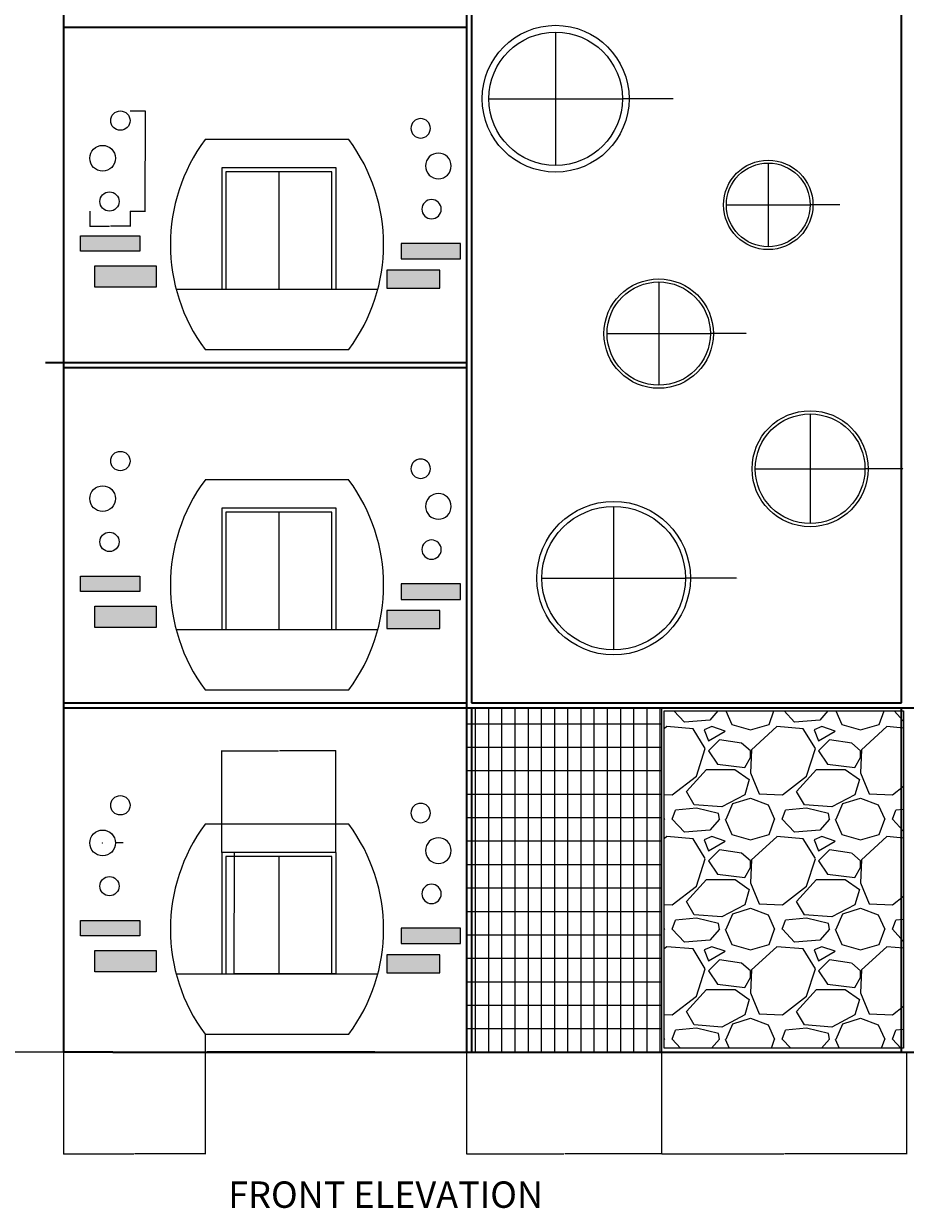
# Model space of a CAD drawing. Units: inches. Extents: x 328 to 2318, y 647 to 2548.
# Tile 2 of 5: x 1040 to 1841, y 647 to 1724. Entities that reach past the tile are written whole.
import ezdxf

# ---------------------------------------------------------------- set-up
doc = ezdxf.new("R2010")
doc.units = ezdxf.units.IN
doc.header["$MEASUREMENT"] = 0
for name, color, linetype, lineweight in [('A-ANNO-DIMS', 2, 'Continuous', 18), ('A-ANNO-TEXT', 7, 'Continuous', 25), ('A-ELEV', 7, 'Continuous', 35), ('A-ELEV-CLAD', 7, 'Continuous', 25), ('A-ELEV-ORNM', 7, 'Continuous', 18), ('A-ELEV-PATT', 8, 'Continuous', 13), ('A-GLAZ', 4, 'Continuous', 25)]:
    doc.layers.add(name, color=color, linetype=linetype, lineweight=lineweight)
doc.layers.add('A-ELEV-ORNM-PATT', color=18, linetype='Continuous', lineweight=13, true_color=0x000000)
doc.styles.get("Standard").update_dxf_attribs({"font": 'arial.ttf'})
doc.dimstyles.get("Standard").update_dxf_attribs({"dimtxt": 0.18, "dimasz": 0.18, "dimexe": 0.18, "dimexo": 0.0625, "dimgap": 0.09, "dimtad": 0, "dimtih": 1, "dimtoh": 1, "dimdec": 4, "dimzin": 0, "dimdsep": 46, "dimtxsty": 'Standard', "dimcen": 0.09, "dimadec": 0, "dimazin": 0, "dimtfac": 1, "dimtdec": 4, "dimtofl": 0, "dimtmove": 0, "dimatfit": 3, "dimfxl": 1, "dimtolj": 1, "dimtzin": 0, "dimarcsym": 0})

# ---------------------------------------------------------------- blocks, each defined once
blk = doc.blocks.new('WIN-ELEV-CURVED-SURROUND')
for p, q in [((162.1, 190.7), (31.6, 190.7)), ((98.6, 161.4), (98.6, 54.8)), ((5.2, 54.8), (188.5, 54.8)), ((31.6, 0), (162.1, 0))]:
    blk.add_line(p, q)
for points in [[(150.5, 54.8), (150.5, 165.1), (46.8, 165.1), (46.8, 54.8)], [(146.8, 54.8), (146.8, 161.4), (50.5, 161.4), (50.5, 54.8)]]:
    blk.add_lwpolyline(points)
for centre, start, end in [((159.8, 95.3), 143.3588, 216.6412), ((33.9, 95.3), 323.3588, 36.6412)]:
    blk.add_arc(centre, 159.8, start, end)
blk = doc.blocks.new('FACADE-THREE-ROUNDELS')
for centre, radius in [((27.8, 82.3), 8.8), ((11.7, 48.1), 11.7), ((17.9, 8.8), 8.77)]:
    blk.add_circle(centre, radius)
blk = doc.blocks.new('*D11')
at = {"layer": 'A-ANNO-DIMS', "color": 0, "lineweight": -2, "transparency": 16777216}
for p, q in [((1137.1, 1644.2), (1150.9, 1644.2)), ((1150.7, 1644), (1150.7, 1598.9)), ((1150.7, 1553.3), (1150.7, 1598.5)), ((1137.1, 1553.1), (1150.9, 1553.1))]:
    blk.add_line(p, q, dxfattribs=at)
at = {"layer": 'A-ANNO-DIMS', "color": 0, "transparency": 16777216}
for points in [[(1150.7, 1644), (1150.7, 1644), (1150.7, 1644.2)], [(1150.7, 1553.3), (1150.7, 1553.3), (1150.7, 1553.1)]]:
    blk.add_solid(points, dxfattribs=at)
at = {"layer": 'Defpoints', "color": 0, "transparency": 16777216}
for p in [(1137, 1644.2), (1150.7, 1644.2), (1137, 1553.1)]:
    blk.add_point(p, dxfattribs=at)
at = {"layer": 'A-ANNO-DIMS', "color": 0, "transparency": 16777216, "insert": (1150.7, 1598.7), "char_height": 0.18, "attachment_point": 5}
blk.add_mtext('\\A1;ROUNDELS 91 TYP.', dxfattribs=at)
blk = doc.blocks.new('*D12')
at = {"layer": 'A-ANNO-DIMS', "color": 0, "lineweight": -2, "transparency": 16777216}
for p, q in [((1100.4, 1553.1), (1100.4, 1539.3)), ((1137, 1553.1), (1137, 1539.3)), ((1100.6, 1539.5), (1118.2, 1539.5)), ((1136.8, 1539.5), (1119.2, 1539.5))]:
    blk.add_line(p, q, dxfattribs=at)
at = {"layer": 'A-ANNO-DIMS', "color": 0, "transparency": 16777216}
for points in [[(1100.6, 1539.5), (1100.6, 1539.5), (1100.4, 1539.5)], [(1136.8, 1539.5), (1136.8, 1539.5), (1137, 1539.5)]]:
    blk.add_solid(points, dxfattribs=at)
at = {"layer": 'Defpoints', "color": 0, "transparency": 16777216}
for p in [(1100.4, 1553.1), (1137, 1553.1), (1137, 1539.5)]:
    blk.add_point(p, dxfattribs=at)
at = {"layer": 'A-ANNO-DIMS', "color": 0, "transparency": 16777216, "insert": (1118.7, 1539.5), "char_height": 0.18, "attachment_point": 5}
blk.add_mtext('\\A1;37 TYP.', dxfattribs=at)
blk = doc.blocks.new('*D40')
at = {"layer": 'A-ANNO-DIMS', "color": 0, "lineweight": -2, "transparency": 16777216}
for p, q in [((1362.3, 2455.5), (967.6, 2455.5)), ((967.8, 2455.4), (967.8, 1622.3)), ((967.8, 789), (967.8, 1622)), ((1076.4, 788.8), (967.6, 788.8))]:
    blk.add_line(p, q, dxfattribs=at)
at = {"layer": 'A-ANNO-DIMS', "color": 0, "transparency": 16777216}
for points in [[(967.8, 2455.4), (967.9, 2455.4), (967.8, 2455.5)], [(967.8, 789), (967.9, 789), (967.8, 788.8)]]:
    blk.add_solid(points, dxfattribs=at)
at = {"layer": 'Defpoints', "color": 0, "transparency": 16777216}
for p in [(967.8, 2455.5), (1362.4, 2455.5), (1076.4, 788.8)]:
    blk.add_point(p, dxfattribs=at)
at = {"layer": 'A-ANNO-DIMS', "color": 0, "transparency": 16777216, "insert": (967.8, 1622.2), "char_height": 0.18, "attachment_point": 5}
blk.add_mtext('\\A1;1666.7', dxfattribs=at)
blk = doc.blocks.new('*D53')
at = {"layer": 'A-ANNO-DIMS', "color": 0, "lineweight": -2, "transparency": 16777216}
for p, q in [((1205.2, 805.1), (1205.2, 696.2)), ((1076.4, 788.7), (1076.4, 696.2)), ((1076.6, 696.3), (1140.4, 696.3)), ((1205, 696.3), (1141.2, 696.3))]:
    blk.add_line(p, q, dxfattribs=at)
at = {"layer": 'A-ANNO-DIMS', "color": 0, "transparency": 16777216}
for points in [[(1076.6, 696.4), (1076.6, 696.3), (1076.4, 696.3)], [(1205, 696.4), (1205, 696.3), (1205.2, 696.3)]]:
    blk.add_solid(points, dxfattribs=at)
at = {"layer": 'Defpoints', "color": 0, "transparency": 16777216}
for p in [(1205.2, 805.2), (1076.4, 788.8), (1205.2, 696.3)]:
    blk.add_point(p, dxfattribs=at)
at = {"layer": 'A-ANNO-DIMS', "color": 0, "transparency": 16777216, "insert": (1140.8, 696.3), "char_height": 0.18, "attachment_point": 5}
blk.add_mtext('\\A1;128.8', dxfattribs=at)
blk = doc.blocks.new('*D56')
at = {"layer": 'A-ANNO-DIMS', "color": 0, "lineweight": -2, "transparency": 16777216}
for p, q in [((1442.8, 788.7), (1442.8, 696.2)), ((1620, 788.7), (1620, 696.2)), ((1443, 696.3), (1531, 696.3)), ((1619.9, 696.3), (1531.9, 696.3))]:
    blk.add_line(p, q, dxfattribs=at)
at = {"layer": 'A-ANNO-DIMS', "color": 0, "transparency": 16777216}
for points in [[(1443, 696.4), (1443, 696.3), (1442.8, 696.3)], [(1619.9, 696.4), (1619.9, 696.3), (1620, 696.3)]]:
    blk.add_solid(points, dxfattribs=at)
at = {"layer": 'Defpoints', "color": 0, "transparency": 16777216}
for p in [(1442.8, 788.8), (1620, 788.8), (1442.8, 696.3)]:
    blk.add_point(p, dxfattribs=at)
at = {"layer": 'A-ANNO-DIMS', "color": 0, "transparency": 16777216, "insert": (1531.4, 696.3), "char_height": 0.18, "attachment_point": 5}
blk.add_mtext('\\A1;177.24', dxfattribs=at)
blk = doc.blocks.new('*D57')
at = {"layer": 'A-ANNO-DIMS', "color": 0, "lineweight": -2, "transparency": 16777216}
for p, q in [((1620, 788.7), (1620, 696.2)), ((1842.4, 788.7), (1842.4, 696.2)), ((1620.2, 696.3), (1730.9, 696.3)), ((1842.3, 696.3), (1731.6, 696.3))]:
    blk.add_line(p, q, dxfattribs=at)
at = {"layer": 'A-ANNO-DIMS', "color": 0, "transparency": 16777216}
for points in [[(1620.2, 696.4), (1620.2, 696.3), (1620, 696.3)], [(1842.3, 696.4), (1842.3, 696.3), (1842.4, 696.3)]]:
    blk.add_solid(points, dxfattribs=at)
at = {"layer": 'Defpoints', "color": 0, "transparency": 16777216}
for p in [(1620, 788.8), (1842.4, 788.8), (1620, 696.3)]:
    blk.add_point(p, dxfattribs=at)
at = {"layer": 'A-ANNO-DIMS', "color": 0, "transparency": 16777216, "insert": (1731.2, 696.3), "char_height": 0.18, "attachment_point": 5}
blk.add_mtext('\\A1;222.4', dxfattribs=at)
blk = doc.blocks.new('*D58')
at = {"layer": 'A-ANNO-DIMS', "color": 0, "lineweight": -2, "transparency": 16777216}
for p, q in [((1220.4, 970.3), (1220.4, 1062.9)), ((1220.6, 1062.7), (1271.8, 1062.7)), ((1323.9, 1062.7), (1272.7, 1062.7)), ((1324.1, 970.3), (1324.1, 1062.9))]:
    blk.add_line(p, q, dxfattribs=at)
at = {"layer": 'A-ANNO-DIMS', "color": 0, "transparency": 16777216}
for points in [[(1220.6, 1062.8), (1220.6, 1062.7), (1220.4, 1062.7)], [(1323.9, 1062.8), (1323.9, 1062.7), (1324.1, 1062.7)]]:
    blk.add_solid(points, dxfattribs=at)
at = {"layer": 'Defpoints', "color": 0, "transparency": 16777216}
for p in [(1324.1, 1062.7), (1220.4, 970.3), (1324.1, 970.3)]:
    blk.add_point(p, dxfattribs=at)
at = {"layer": 'A-ANNO-DIMS', "color": 0, "transparency": 16777216, "insert": (1272.3, 1062.7), "char_height": 0.18, "attachment_point": 5}
blk.add_mtext('\\A1;103.68', dxfattribs=at)
blk = doc.blocks.new('*D59')
at = {"layer": 'A-ANNO-DIMS', "color": 0, "lineweight": -2, "transparency": 16777216}
for p, q in [((1324.1, 970.3), (1231.5, 970.3)), ((1231.7, 970.1), (1231.7, 915.3)), ((1231.7, 860.2), (1231.7, 915)), ((1324.1, 860), (1231.5, 860))]:
    blk.add_line(p, q, dxfattribs=at)
at = {"layer": 'A-ANNO-DIMS', "color": 0, "transparency": 16777216}
for points in [[(1231.6, 970.1), (1231.7, 970.1), (1231.7, 970.3)], [(1231.6, 860.2), (1231.7, 860.2), (1231.7, 860)]]:
    blk.add_solid(points, dxfattribs=at)
at = {"layer": 'Defpoints', "color": 0, "transparency": 16777216}
for p in [(1231.7, 970.3), (1324.1, 970.3), (1324.1, 860)]:
    blk.add_point(p, dxfattribs=at)
at = {"layer": 'A-ANNO-DIMS', "color": 0, "transparency": 16777216, "insert": (1231.7, 915.1), "char_height": 0.18, "attachment_point": 5}
blk.add_mtext('\\A1;110.26', dxfattribs=at)
blk = doc.blocks.new('*D69')
at = {"layer": 'A-ANNO-DIMS', "color": 0, "lineweight": -2, "transparency": 16777216}
for p, q in [((1112, 978.9), (1112.2, 978.9)), ((1112.1, 978.8), (1112.1, 979)), ((1130.8, 978.9), (1124, 978.9))]:
    blk.add_line(p, q, dxfattribs=at)
at = {"layer": 'A-ANNO-DIMS', "color": 0, "transparency": 16777216}
blk.add_solid([(1124, 979), (1124, 978.9), (1123.8, 978.9)], dxfattribs=at)
at = {"layer": 'Defpoints', "color": 0, "transparency": 16777216}
for p in [(1100.4, 978.9), (1123.8, 978.9)]:
    blk.add_point(p, dxfattribs=at)
at = {"layer": 'A-ANNO-DIMS', "color": 0, "transparency": 16777216, "insert": (1131.6, 978.9), "char_height": 0.18, "attachment_point": 5}
blk.add_mtext('\\A1;16X ∅23.394', dxfattribs=at)
blk = doc.blocks.new('*D74')
at = {"layer": 'A-ANNO-DIMS', "color": 0, "lineweight": -2, "transparency": 16777216}
for p, q in [((1523.6, 1655.4), (1523.8, 1655.4)), ((1523.7, 1655.3), (1523.7, 1655.4)), ((1630.4, 1655.4), (1590.6, 1655.4))]:
    blk.add_line(p, q, dxfattribs=at)
at = {"layer": 'A-ANNO-DIMS', "color": 0, "transparency": 16777216}
blk.add_solid([(1590.6, 1655.4), (1590.6, 1655.3), (1590.4, 1655.4)], dxfattribs=at)
at = {"layer": 'Defpoints', "color": 0, "transparency": 16777216}
for p in [(1457, 1655.4), (1590.4, 1655.4)]:
    blk.add_point(p, dxfattribs=at)
at = {"layer": 'A-ANNO-DIMS', "color": 0, "transparency": 16777216, "insert": (1631, 1655.4), "char_height": 0.18, "attachment_point": 5}
blk.add_mtext('\\A1;∅133.42', dxfattribs=at)
blk = doc.blocks.new('*D75')
at = {"layer": 'A-ANNO-DIMS', "color": 0, "lineweight": -2, "transparency": 16777216}
for p, q in [((1523.6, 1655.4), (1523.8, 1655.4)), ((1523.7, 1655.3), (1523.7, 1655.4)), ((1620.7, 1655.4), (1584.5, 1655.4))]:
    blk.add_line(p, q, dxfattribs=at)
at = {"layer": 'A-ANNO-DIMS', "color": 0, "transparency": 16777216}
blk.add_solid([(1584.5, 1655.4), (1584.5, 1655.3), (1584.3, 1655.4)], dxfattribs=at)
at = {"layer": 'Defpoints', "color": 0, "transparency": 16777216}
for p in [(1463.1, 1655.4), (1584.3, 1655.4)]:
    blk.add_point(p, dxfattribs=at)
at = {"layer": 'A-ANNO-DIMS', "color": 0, "transparency": 16777216, "insert": (1621.2, 1655.4), "char_height": 0.18, "attachment_point": 5}
blk.add_mtext('\\A1;∅121.25', dxfattribs=at)
blk = doc.blocks.new('*D76')
at = {"layer": 'A-ANNO-DIMS', "color": 0, "lineweight": -2, "transparency": 16777216}
for p, q in [((1617.2, 1441.9), (1617.4, 1441.9)), ((1617.3, 1441.8), (1617.3, 1442)), ((1696.9, 1441.9), (1667.2, 1441.9))]:
    blk.add_line(p, q, dxfattribs=at)
at = {"layer": 'A-ANNO-DIMS', "color": 0, "transparency": 16777216}
blk.add_solid([(1667.2, 1441.9), (1667.2, 1441.8), (1667.1, 1441.9)], dxfattribs=at)
at = {"layer": 'Defpoints', "color": 0, "transparency": 16777216}
for p in [(1567.6, 1441.9), (1667.1, 1441.9)]:
    blk.add_point(p, dxfattribs=at)
at = {"layer": 'A-ANNO-DIMS', "color": 0, "transparency": 16777216, "insert": (1697.4, 1441.9), "char_height": 0.18, "attachment_point": 5}
blk.add_mtext('\\A1;∅99.45', dxfattribs=at)
blk = doc.blocks.new('*D77')
at = {"layer": 'A-ANNO-DIMS', "color": 0, "lineweight": -2, "transparency": 16777216}
for p, q in [((1617.2, 1441.9), (1617.4, 1441.9)), ((1617.3, 1441.8), (1617.3, 1442)), ((1692.4, 1441.9), (1664.5, 1441.9))]:
    blk.add_line(p, q, dxfattribs=at)
at = {"layer": 'A-ANNO-DIMS', "color": 0, "transparency": 16777216}
blk.add_solid([(1664.5, 1441.9), (1664.5, 1441.8), (1664.3, 1441.9)], dxfattribs=at)
at = {"layer": 'Defpoints', "color": 0, "transparency": 16777216}
for p in [(1570.4, 1441.9), (1664.3, 1441.9)]:
    blk.add_point(p, dxfattribs=at)
at = {"layer": 'A-ANNO-DIMS', "color": 0, "transparency": 16777216, "insert": (1692.9, 1441.9), "char_height": 0.18, "attachment_point": 5}
blk.add_mtext('\\A1;∅93.88', dxfattribs=at)
blk = doc.blocks.new('*D84')
at = {"layer": 'A-ANNO-DIMS', "color": 0, "lineweight": -2, "transparency": 16777216}
for p, q in [((1716.8, 1558.8), (1716.8, 1558.9)), ((1716.8, 1558.8), (1716.9, 1558.8)), ((1781.9, 1558.8), (1757.7, 1558.8))]:
    blk.add_line(p, q, dxfattribs=at)
at = {"layer": 'A-ANNO-DIMS', "color": 0, "transparency": 16777216}
blk.add_solid([(1757.7, 1558.9), (1757.7, 1558.8), (1757.5, 1558.8)], dxfattribs=at)
at = {"layer": 'Defpoints', "color": 0, "transparency": 16777216}
for p in [(1676.2, 1558.8), (1757.5, 1558.8)]:
    blk.add_point(p, dxfattribs=at)
at = {"layer": 'A-ANNO-DIMS', "color": 0, "transparency": 16777216, "insert": (1782.4, 1558.8), "char_height": 0.18, "attachment_point": 5}
blk.add_mtext('\\A1;∅81.27', dxfattribs=at)
blk = doc.blocks.new('*D85')
at = {"layer": 'A-ANNO-DIMS', "color": 0, "lineweight": -2, "transparency": 16777216}
for p, q in [((1716.8, 1558.8), (1716.8, 1558.9)), ((1716.8, 1558.8), (1716.9, 1558.8)), ((1777.7, 1558.8), (1755, 1558.8))]:
    blk.add_line(p, q, dxfattribs=at)
at = {"layer": 'A-ANNO-DIMS', "color": 0, "transparency": 16777216}
blk.add_solid([(1755, 1558.9), (1755, 1558.8), (1754.9, 1558.8)], dxfattribs=at)
at = {"layer": 'Defpoints', "color": 0, "transparency": 16777216}
for p in [(1678.8, 1558.8), (1754.9, 1558.8)]:
    blk.add_point(p, dxfattribs=at)
at = {"layer": 'A-ANNO-DIMS', "color": 0, "transparency": 16777216, "insert": (1778.2, 1558.8), "char_height": 0.18, "attachment_point": 5}
blk.add_mtext('\\A1;∅76.06', dxfattribs=at)
blk = doc.blocks.new('*D86')
at = {"layer": 'A-ANNO-DIMS', "color": 0, "lineweight": -2, "transparency": 16777216}
for p, q in [((1576.3, 1219.6), (1576.4, 1219.6)), ((1576.4, 1219.5), (1576.4, 1219.7)), ((1688, 1219.6), (1646.3, 1219.6))]:
    blk.add_line(p, q, dxfattribs=at)
at = {"layer": 'A-ANNO-DIMS', "color": 0, "transparency": 16777216}
blk.add_solid([(1646.3, 1219.6), (1646.3, 1219.6), (1646.1, 1219.6)], dxfattribs=at)
at = {"layer": 'Defpoints', "color": 0, "transparency": 16777216}
for p in [(1506.6, 1219.6), (1646.1, 1219.6)]:
    blk.add_point(p, dxfattribs=at)
at = {"layer": 'A-ANNO-DIMS', "color": 0, "transparency": 16777216, "insert": (1688.6, 1219.6), "char_height": 0.18, "attachment_point": 5}
blk.add_mtext('\\A1;∅139.55', dxfattribs=at)
blk = doc.blocks.new('*D87')
at = {"layer": 'A-ANNO-DIMS', "color": 0, "lineweight": -2, "transparency": 16777216}
for p, q in [((1576.3, 1219.6), (1576.4, 1219.6)), ((1576.4, 1219.5), (1576.4, 1219.7)), ((1680.7, 1219.6), (1641.8, 1219.6))]:
    blk.add_line(p, q, dxfattribs=at)
at = {"layer": 'A-ANNO-DIMS', "color": 0, "transparency": 16777216}
blk.add_solid([(1641.8, 1219.6), (1641.8, 1219.6), (1641.6, 1219.6)], dxfattribs=at)
at = {"layer": 'Defpoints', "color": 0, "transparency": 16777216}
for p in [(1511.1, 1219.6), (1641.6, 1219.6)]:
    blk.add_point(p, dxfattribs=at)
at = {"layer": 'A-ANNO-DIMS', "color": 0, "transparency": 16777216, "insert": (1681.3, 1219.6), "char_height": 0.18, "attachment_point": 5}
blk.add_mtext('\\A1;∅130.43', dxfattribs=at)
blk = doc.blocks.new('*D88')
at = {"layer": 'A-ANNO-DIMS', "color": 0, "lineweight": -2, "transparency": 16777216}
for p, q in [((1754.8, 1319), (1755, 1319)), ((1754.9, 1318.9), (1754.9, 1319.1)), ((1839.2, 1319), (1807.8, 1319))]:
    blk.add_line(p, q, dxfattribs=at)
at = {"layer": 'A-ANNO-DIMS', "color": 0, "transparency": 16777216}
blk.add_solid([(1807.8, 1319.1), (1807.8, 1319), (1807.6, 1319)], dxfattribs=at)
at = {"layer": 'Defpoints', "color": 0, "transparency": 16777216}
for p in [(1702.2, 1319), (1807.6, 1319)]:
    blk.add_point(p, dxfattribs=at)
at = {"layer": 'A-ANNO-DIMS', "color": 0, "transparency": 16777216, "insert": (1839.8, 1319), "char_height": 0.18, "attachment_point": 5}
blk.add_mtext('\\A1;∅105.45', dxfattribs=at)
blk = doc.blocks.new('*D89')
at = {"layer": 'A-ANNO-DIMS', "color": 0, "lineweight": -2, "transparency": 16777216}
for p, q in [((1754.8, 1319), (1755, 1319)), ((1754.9, 1318.9), (1754.9, 1319.1)), ((1834.6, 1319), (1804.9, 1319))]:
    blk.add_line(p, q, dxfattribs=at)
at = {"layer": 'A-ANNO-DIMS', "color": 0, "transparency": 16777216}
blk.add_solid([(1804.9, 1319.1), (1804.9, 1319), (1804.7, 1319)], dxfattribs=at)
at = {"layer": 'Defpoints', "color": 0, "transparency": 16777216}
for p in [(1705, 1319), (1804.7, 1319)]:
    blk.add_point(p, dxfattribs=at)
at = {"layer": 'A-ANNO-DIMS', "color": 0, "transparency": 16777216, "insert": (1835.1, 1319), "char_height": 0.18, "attachment_point": 5}
blk.add_mtext('\\A1;∅99.7', dxfattribs=at)

msp = doc.modelspace()

# ---------------------------------------------------------------- hatches: boundary and pattern name
at = {"layer": 'A-ELEV-ORNM-PATT'}
h = msp.add_hatch(color=256, dxfattribs=at)
h.dxf.hatch_style = 1
h.paths.add_polyline_path([(1160.8736, 1194.017), (1104.946, 1194.017), (1104.946, 1174.8467), (1160.8736, 1174.8467)])
h.paths.add_polyline_path([(1145.9162, 1221.3103), (1091.9395, 1221.3103), (1091.9395, 1207.3388), (1145.9162, 1207.3388)])
h.paths.add_polyline_path([(1418.337, 1190.1501), (1370.4156, 1190.1501), (1370.4156, 1173.7241), (1418.337, 1173.7241)])
h.paths.add_polyline_path([(1437.3105, 1214.299), (1383.3339, 1214.299), (1383.3339, 1200.3274), (1437.3105, 1200.3274)])
h.paths.add_polyline_path([(1418.337, 1499.5227), (1370.4156, 1499.5227), (1370.4156, 1483.0967), (1418.337, 1483.0967)])
h.paths.add_polyline_path([(1437.3105, 1523.6716), (1383.3339, 1523.6716), (1383.3339, 1509.7), (1437.3105, 1509.7)])
h.paths.add_polyline_path([(1145.9162, 1530.683), (1091.9395, 1530.683), (1091.9395, 1516.7114), (1145.9162, 1516.7114)])
h.paths.add_polyline_path([(1160.8736, 1503.3896), (1104.946, 1503.3896), (1104.946, 1484.2194), (1160.8736, 1484.2194)])
h.paths.add_polyline_path([(1160.8736, 1812.7623), (1104.946, 1812.7623), (1104.946, 1793.592), (1160.8736, 1793.592)])
h.paths.add_polyline_path([(1145.9162, 1840.0556), (1091.9395, 1840.0556), (1091.9395, 1826.084), (1145.9162, 1826.084)])
h.paths.add_polyline_path([(1437.3105, 1833.0442), (1383.3339, 1833.0442), (1383.3339, 1819.0726), (1437.3105, 1819.0726)])
h.paths.add_polyline_path([(1418.337, 1808.8953), (1370.4156, 1808.8953), (1370.4156, 1792.4693), (1418.337, 1792.4693)])
h.paths.add_polyline_path([(1145.9162, 908.3867), (1091.9395, 908.3867), (1091.9395, 894.4151), (1145.9162, 894.4151)])
h.paths.add_polyline_path([(1160.8736, 881.0933), (1104.946, 881.0933), (1104.946, 861.923), (1160.8736, 861.923)])
h.paths.add_polyline_path([(1418.337, 877.2264), (1370.4156, 877.2264), (1370.4156, 860.8004), (1418.337, 860.8004)])
h.paths.add_polyline_path([(1437.3105, 901.3753), (1383.3339, 901.3753), (1383.3339, 887.4037), (1437.3105, 887.4037)])
h.paths.add_polyline_path([(1926.897, 881.0933), (1870.9694, 881.0933), (1870.9694, 861.923), (1926.897, 861.923)])
h.paths.add_polyline_path([(1911.9396, 908.3867), (1857.9629, 908.3867), (1857.9629, 894.4151), (1911.9396, 894.4151)])
h.paths.add_polyline_path([(2184.3603, 877.2264), (2136.439, 877.2264), (2136.439, 860.8004), (2184.3603, 860.8004)])
h.paths.add_polyline_path([(2203.3339, 901.3753), (2149.3572, 901.3753), (2149.3572, 887.4037), (2203.3339, 887.4037)])
h.paths.add_polyline_path([(2184.3603, 1190.1501), (2136.439, 1190.1501), (2136.439, 1173.7241), (2184.3603, 1173.7241)])
h.paths.add_polyline_path([(2203.3339, 1214.299), (2149.3572, 1214.299), (2149.3572, 1200.3274), (2203.3339, 1200.3274)])
h.paths.add_polyline_path([(1911.9396, 1221.3103), (1857.9629, 1221.3103), (1857.9629, 1207.3388), (1911.9396, 1207.3388)])
h.paths.add_polyline_path([(1926.897, 1194.017), (1870.9694, 1194.017), (1870.9694, 1174.8467), (1926.897, 1174.8467)])
h.paths.add_polyline_path([(1926.897, 1503.3896), (1870.9694, 1503.3896), (1870.9694, 1484.2194), (1926.897, 1484.2194)])
h.paths.add_polyline_path([(1911.9396, 1530.683), (1857.9629, 1530.683), (1857.9629, 1516.7114), (1911.9396, 1516.7114)])
h.paths.add_polyline_path([(2184.3603, 1499.5227), (2136.439, 1499.5227), (2136.439, 1483.0967), (2184.3603, 1483.0967)])
h.paths.add_polyline_path([(2203.3339, 1523.6716), (2149.3572, 1523.6716), (2149.3572, 1509.7), (2203.3339, 1509.7)])
h.paths.add_polyline_path([(1926.897, 1812.7623), (1870.9694, 1812.7623), (1870.9694, 1793.592), (1926.897, 1793.592)])
h.paths.add_polyline_path([(1911.9396, 1840.0556), (1857.9629, 1840.0556), (1857.9629, 1826.084), (1911.9396, 1826.084)])
h.paths.add_polyline_path([(2184.3603, 1808.8953), (2136.439, 1808.8953), (2136.439, 1792.4693), (2184.3603, 1792.4693)])
h.paths.add_polyline_path([(2203.3339, 1833.0442), (2149.3572, 1833.0442), (2149.3572, 1819.0726), (2203.3339, 1819.0726)])
at = {"layer": 'A-ELEV-PATT'}
h = msp.add_hatch(dxfattribs=at)
h.set_pattern_fill('ANSI31', color=256, scale=95.928, angle=45, style=0)
h.paths.add_polyline_path([(1442.8075, 788.791), (1620.0467, 788.791), (1620.0467, 1101.7147), (1442.8075, 1101.7147)])
h = msp.add_hatch(dxfattribs=at)
h.set_pattern_fill('ANSI31', color=256, scale=170.557, angle=-45, style=0)
h.paths.add_polyline_path([(1442.8075, 788.791), (1620.0467, 788.791), (1620.0467, 1101.7147), (1442.8075, 1101.7147)])
h = msp.add_hatch(dxfattribs=at)
h.set_pattern_fill('GRAVEL', color=256, scale=100)
h.paths.add_polyline_path([(1839.8727, 1098.9753), (1622.4148, 1098.9753), (1622.4148, 792.342), (1839.8727, 792.342)])

# ---------------------------------------------------------------- linework, layer by layer
at = {"layer": 'A-ELEV'}
for p, q in [((1442.8075, 2242.4288), (1442.8075, 1101.7147)), ((1447.3872, 2242.4288), (1447.3872, 1106.2944)), ((1837.8703, 1106.2944), (1837.8703, 2242.4288)), ((1076.4266, 2069.5914), (1076.4266, 788.791)), ((1076.4266, 1720.4599), (1442.8075, 1720.4599)), ((1060.276, 1415.667), (1442.8075, 1415.667)), ((1076.4266, 1411.0873), (1442.8075, 1411.0873)), ((1076.4266, 1106.2944), (1442.8075, 1106.2944)), ((1076.4266, 1101.7147), (2224.9815, 1101.7147)), ((1442.8075, 1101.7147), (1442.8075, 788.791)), ((1447.3872, 1106.2944), (1837.8703, 1106.2944)), ((1447.3872, 1101.7147), (1447.3872, 788.791)), ((1837.8703, 788.791), (1837.8703, 1101.7147)), ((1121.2827, 788.791), (1076.4266, 788.791)), ((1121.2827, 788.791), (2224.9815, 788.791))]:
    msp.add_line(p, q, dxfattribs=at)
for points in [[(1359.5368, 788.791), (1207.1846, 788.791)], [(1224.958, 788.791), (1345.9577, 788.791)]]:
    msp.add_lwpolyline(points, dxfattribs=at)
at = {"layer": 'A-ELEV-CLAD'}
for p, q in [((1620.0467, 788.791), (1620.0467, 1101.7147)), ((1442.8075, 788.791), (1620.0467, 788.791))]:
    msp.add_line(p, q, dxfattribs=at)
msp.add_lwpolyline([(1622.4148, 1098.9753), (1839.8727, 1098.9753), (1839.8727, 792.342), (1622.4148, 792.342)], close=True, dxfattribs=at)
at = {"layer": 'A-ELEV-ORNM'}
for points in [[(1091.9395, 1530.683), (1145.9162, 1530.683), (1145.9162, 1516.7114), (1091.9395, 1516.7114)], [(1437.3105, 1523.6716), (1383.3339, 1523.6716), (1383.3339, 1509.7), (1437.3105, 1509.7)], [(1104.946, 1503.3896), (1160.8736, 1503.3896), (1160.8736, 1484.2194), (1104.946, 1484.2194)], [(1418.337, 1499.5227), (1370.4156, 1499.5227), (1370.4156, 1483.0967), (1418.337, 1483.0967)], [(1091.9395, 1221.3103), (1145.9162, 1221.3103), (1145.9162, 1207.3388), (1091.9395, 1207.3388)], [(1437.3105, 1214.299), (1383.3339, 1214.299), (1383.3339, 1200.3274), (1437.3105, 1200.3274)], [(1104.946, 1194.017), (1160.8736, 1194.017), (1160.8736, 1174.8467), (1104.946, 1174.8467)], [(1418.337, 1190.1501), (1370.4156, 1190.1501), (1370.4156, 1173.7241), (1418.337, 1173.7241)], [(1091.9395, 908.3867), (1145.9162, 908.3867), (1145.9162, 894.4151), (1091.9395, 894.4151)], [(1437.3105, 901.3753), (1383.3339, 901.3753), (1383.3339, 887.4037), (1437.3105, 887.4037)], [(1104.946, 881.0933), (1160.8736, 881.0933), (1160.8736, 861.923), (1104.946, 861.923)], [(1418.337, 877.2264), (1370.4156, 877.2264), (1370.4156, 860.8004), (1418.337, 860.8004)]]:
    msp.add_lwpolyline(points, close=True, dxfattribs=at)
at = {"layer": 'A-GLAZ'}
for p, q in [((1523.6794, 1715.9816), (1523.6794, 1594.7308)), ((1463.054, 1655.3562), (1584.3048, 1655.3562)), ((1716.8405, 1596.8754), (1716.8405, 1520.8187)), ((1678.8121, 1558.8471), (1754.8688, 1558.8471)), ((1617.3332, 1488.8052), (1617.3332, 1394.9272)), ((1570.3942, 1441.8662), (1664.2722, 1441.8662)), ((1754.8873, 1368.8864), (1754.8873, 1269.1863)), ((1705.0373, 1319.0364), (1804.7374, 1319.0364)), ((1576.3597, 1284.8181), (1576.3597, 1154.3873)), ((1511.1442, 1219.6027), (1641.5751, 1219.6027))]:
    msp.add_line(p, q, dxfattribs=at)
for centre, radius in [((1523.6794, 1655.3562), 66.7079), ((1523.6794, 1655.3562), 60.6254), ((1716.8405, 1558.8471), 40.6364), ((1716.8405, 1558.8471), 38.0284), ((1617.3332, 1441.8662), 49.725), ((1617.3332, 1441.8662), 46.939), ((1754.8873, 1319.0364), 52.7227), ((1754.8873, 1319.0364), 49.8501), ((1576.3597, 1219.6027), 69.776), ((1576.3597, 1219.6027), 65.2154)]:
    msp.add_circle(centre, radius, dxfattribs=at)

# ---------------------------------------------------------------- block references
at = {"layer": 'A-ELEV-ORNM'}
for p in [(1100.4017, 1553.1455), (1100.4017, 1243.7728), (1100.4017, 930.8492)]:
    msp.add_blockref('FACADE-THREE-ROUNDELS', p, dxfattribs=at)
at = {"layer": 'A-ELEV-ORNM', "extrusion": (0, 0, -1), "zscale": -1}
for p in [(-1428.8484, 1546.1341), (-1428.8484, 1236.7615), (-1428.8484, 923.8378)]:
    msp.add_blockref('FACADE-THREE-ROUNDELS', p, dxfattribs=at)
at = {"layer": 'A-GLAZ'}
for p in [(1173.6494, 1427.5026), (1173.6494, 1118.13), (1173.6494, 805.2063)]:
    msp.add_blockref('WIN-ELEV-CURVED-SURROUND', p, dxfattribs=at)

# ---------------------------------------------------------------- texts
at = {"layer": 'A-ANNO-TEXT'}
msp.add_text('FRONT ELEVATION ', height=24, dxfattribs=at).set_placement((1226.1832, 647.2921))

# ---------------------------------------------------------------- dimensions: what is measured, and where the dimension line sits
at = {"layer": 'A-ANNO-DIMS'}
for base, p1, p2, angle, override, picture, middle in [((967.826, 2455.5387), (1076.4266, 788.791), (1362.3871, 2455.5387), 90, {"dimdec": 1, "dimlfac": 1, "dimrnd": 0, "dimzin": 0, "dimdsep": 46, "dimlunit": 2}, '*D40', (967.826, 1622.1648)), ((1231.6769, 970.2726), (1324.1269, 860.0092), (1324.1269, 970.2726), 90, {"dimdec": 2, "dimlfac": 1, "dimrnd": 0, "dimzin": 0, "dimdsep": 46, "dimlunit": 2}, '*D59', (1231.6769, 915.1409)), ((1442.8075, 696.341), (1620.0467, 788.791), (1442.8075, 788.791), 180, {"dimdec": 2, "dimlfac": 1, "dimrnd": 0, "dimzin": 0, "dimdsep": 46, "dimlunit": 2}, '*D56', (1531.4271, 696.341)), ((1620.0467, 696.341), (1842.45, 788.791), (1620.0467, 788.791), 180, {"dimdec": 1, "dimlfac": 1, "dimrnd": 0, "dimzin": 0, "dimdsep": 46, "dimlunit": 2}, '*D57', (1731.2483, 696.341))]:
    dim = msp.add_linear_dim(base=base, p1=p1, p2=p2, angle=angle, dimstyle='Standard', override=override, dxfattribs=at)
    dim.commit()
    dim.dimension.update_dxf_attribs({"geometry": picture, "text_midpoint": middle})
for p1, p2, override, picture, middle in [((1456.9715, 1655.3564), (1590.3873, 1655.356), {"dimdec": 2, "dimlfac": 1, "dimrnd": 0, "dimzin": 0, "dimdsep": 46, "dimlunit": 2}, '*D74', (1630.412, 1655.3559)), ((1463.054, 1655.3564), (1584.3048, 1655.356), {"dimdec": 2, "dimlfac": 1, "dimrnd": 0, "dimzin": 0, "dimdsep": 46, "dimlunit": 2}, '*D75', (1620.6801, 1655.3559)), ((1676.2041, 1558.8471), (1757.4768, 1558.847), {"dimdec": 2, "dimlfac": 1, "dimrnd": 0, "dimzin": 0, "dimdsep": 46, "dimlunit": 2}, '*D84', (1781.8586, 1558.847)), ((1678.8121, 1558.8471), (1754.8688, 1558.847), {"dimdec": 2, "dimlfac": 1, "dimrnd": 0, "dimzin": 0, "dimdsep": 46, "dimlunit": 2}, '*D85', (1777.6858, 1558.847)), ((1567.6083, 1441.8664), (1667.0582, 1441.866), {"dimdec": 2, "dimlfac": 1, "dimrnd": 0, "dimzin": 0, "dimdsep": 46, "dimlunit": 2}, '*D76', (1696.8932, 1441.8659)), ((1570.3942, 1441.8664), (1664.2722, 1441.866), {"dimdec": 2, "dimlfac": 1, "dimrnd": 0, "dimzin": 0, "dimdsep": 46, "dimlunit": 2}, '*D77', (1692.4357, 1441.8659)), ((1702.1647, 1319.0368), (1807.61, 1319.036), {"dimdec": 2, "dimlfac": 1, "dimrnd": 0, "dimzin": 0, "dimdsep": 46, "dimlunit": 2}, '*D88', (1839.2436, 1319.0358)), ((1705.0373, 1319.0368), (1804.7374, 1319.036), {"dimdec": 1, "dimlfac": 1, "dimrnd": 0, "dimzin": 0, "dimdsep": 46, "dimlunit": 2}, '*D89', (1834.6474, 1319.0358)), ((1506.5836, 1219.6024), (1646.1357, 1219.603), {"dimdec": 2, "dimlfac": 1, "dimrnd": 0, "dimzin": 0, "dimdsep": 46, "dimlunit": 2}, '*D86', (1688.0013, 1219.6032)), ((1511.1442, 1219.6024), (1641.5751, 1219.603), {"dimdec": 2, "dimlfac": 1, "dimrnd": 0, "dimzin": 0, "dimdsep": 46, "dimlunit": 2}, '*D87', (1680.7043, 1219.6032))]:
    dim = msp.add_diameter_dim_2p(p1=p1, p2=p2, dimstyle='Standard', override=override, dxfattribs=at)
    dim.commit()
    dim.dimension.update_dxf_attribs({"geometry": picture, "text_midpoint": middle, "dimtype": 163})
dim = msp.add_linear_dim(base=(1150.6895, 1644.2151), p1=(1137.0291, 1553.1455), p2=(1137.0291, 1644.2151), angle=90, text='ROUNDELS <> TYP.', dimstyle='Standard', override={"dimdec": 0, "dimlfac": 1, "dimrnd": 0, "dimzin": 0, "dimdsep": 46, "dimlunit": 2}, dxfattribs=at)
dim.commit()
dim.dimension.update_dxf_attribs({"geometry": '*D11', "text_midpoint": (1150.6895, 1598.6803)})
dim = msp.add_linear_dim(base=(1137.0291, 1539.485), p1=(1100.4017, 1553.1455), p2=(1137.0291, 1553.1455), text='<> TYP.', dimstyle='Standard', override={"dimdec": 0, "dimlfac": 1, "dimrnd": 0, "dimzin": 0, "dimdsep": 46, "dimlunit": 2}, dxfattribs=at)
dim.commit()
dim.dimension.update_dxf_attribs({"geometry": '*D12', "text_midpoint": (1118.7154, 1539.485)})
for base, p1, p2, override, picture, middle in [((1324.1269, 1062.7226), (1220.4489, 970.2726), (1324.1269, 970.2726), {"dimdec": 2, "dimlfac": 1, "dimrnd": 0, "dimzin": 0, "dimdsep": 46, "dimlunit": 2}, '*D58', (1272.2879, 1062.7226)), ((1205.2198, 696.341), (1076.4266, 788.791), (1205.2198, 805.2063), {"dimdec": 1, "dimlfac": 1, "dimrnd": 0, "dimzin": 0, "dimdsep": 46, "dimlunit": 2}, '*D53', (1140.8232, 696.341))]:
    dim = msp.add_linear_dim(base=base, p1=p1, p2=p2, dimstyle='Standard', override=override, dxfattribs=at)
    dim.commit()
    dim.dimension.update_dxf_attribs({"geometry": picture, "text_midpoint": middle})
dim = msp.add_diameter_dim_2p(p1=(1100.4017, 978.9378), p2=(1123.796, 978.937), text='16X <>', dimstyle='Standard', override={"dimdec": 3, "dimlfac": 1, "dimrnd": 0, "dimzin": 0, "dimdsep": 46, "dimlunit": 2}, dxfattribs=at)
dim.commit()
dim.dimension.update_dxf_attribs({"geometry": '*D69', "text_midpoint": (1130.8143, 978.9368), "dimtype": 163})

doc.saveas('drawing.dxf')
